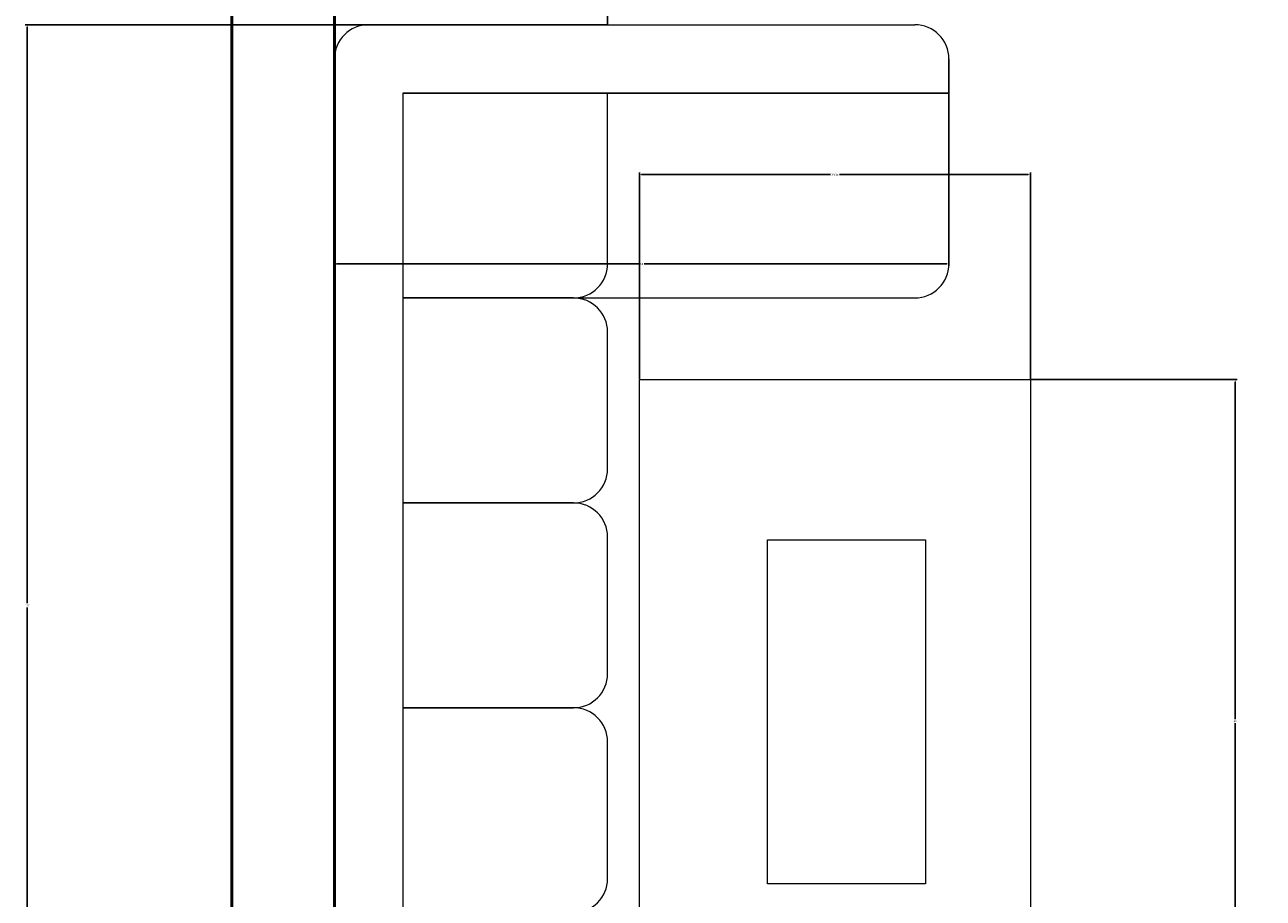
# Model space of a CAD drawing. Units: inches. Extents: x 2621 to 2849, y 2066 to 2463.
# Tile 2 of 28: x 2621 to 2729, y 2123 to 2199. Entities that reach past the tile are written whole.
import ezdxf

# ---------------------------------------------------------------- set-up
doc = ezdxf.new("R2010")
doc.units = ezdxf.units.IN
for name, color, linetype, lineweight in [('A-ANNO-DIMS', 2, 'Continuous', 18), ('A-FLOR-CASE', 9, 'Continuous', 25), ('A-FURN', 8, 'Continuous', 18), ('A-WALL', 7, 'Continuous', 50)]:
    doc.layers.add(name, color=color, linetype=linetype, lineweight=lineweight)
doc.styles.get("Standard").update_dxf_attribs({"font": 'arial.ttf'})
doc.dimstyles.get("Standard").update_dxf_attribs({"dimtxt": 0.18, "dimasz": 0.18, "dimexe": 0.18, "dimexo": 0.0625, "dimgap": 0.09, "dimtad": 0, "dimtih": 1, "dimtoh": 1, "dimdec": 4, "dimzin": 0, "dimdsep": 46, "dimtxsty": 'Standard', "dimcen": 0.09, "dimadec": 0, "dimazin": 0, "dimtfac": 1, "dimtdec": 4, "dimtofl": 0, "dimtmove": 0, "dimatfit": 3, "dimfxl": 1, "dimtolj": 1, "dimtzin": 0, "dimarcsym": 0})

# ---------------------------------------------------------------- blocks, each defined once
blk = doc.blocks.new('*D62')
at = {"layer": 'A-ANNO-DIMS', "color": 0, "lineweight": -2, "transparency": 16777216}
for p, q in [((2647.81, 2199.37), (2620.69, 2199.37)), ((2620.87, 2199.19), (2620.87, 2148.56)), ((2620.87, 2097.55), (2620.87, 2148.19)), ((2647.81, 2097.37), (2620.69, 2097.37))]:
    blk.add_line(p, q, dxfattribs=at)
at = {"layer": 'A-ANNO-DIMS', "color": 0, "transparency": 16777216}
for points in [[(2620.84, 2199.19), (2620.9, 2199.19), (2620.87, 2199.37)], [(2620.84, 2097.55), (2620.9, 2097.55), (2620.87, 2097.37)]]:
    blk.add_solid(points, dxfattribs=at)
at = {"layer": 'Defpoints', "color": 0, "transparency": 16777216}
for p in [(2620.87, 2199.37), (2647.87, 2199.37), (2647.87, 2097.37)]:
    blk.add_point(p, dxfattribs=at)
at = {"layer": 'A-ANNO-DIMS', "color": 0, "transparency": 16777216, "insert": (2620.87, 2148.37), "char_height": 0.18, "attachment_point": 5}
blk.add_mtext('\\A1;102', dxfattribs=at)
blk = doc.blocks.new('*D63')
at = {"layer": 'A-ANNO-DIMS', "color": 0, "lineweight": -2, "transparency": 16777216}
for p, q in [((2647.87, 2196.31), (2647.87, 2178.19)), ((2701.87, 2196.31), (2701.87, 2178.19)), ((2648.05, 2178.37), (2674.65, 2178.37)), ((2701.69, 2178.37), (2675.09, 2178.37))]:
    blk.add_line(p, q, dxfattribs=at)
at = {"layer": 'A-ANNO-DIMS', "color": 0, "transparency": 16777216}
for points in [[(2648.05, 2178.4), (2648.05, 2178.34), (2647.87, 2178.37)], [(2701.69, 2178.4), (2701.69, 2178.34), (2701.87, 2178.37)]]:
    blk.add_solid(points, dxfattribs=at)
at = {"layer": 'Defpoints', "color": 0, "transparency": 16777216}
for p in [(2647.87, 2196.37), (2701.87, 2196.37), (2647.87, 2178.37)]:
    blk.add_point(p, dxfattribs=at)
at = {"layer": 'A-ANNO-DIMS', "color": 0, "transparency": 16777216, "insert": (2674.87, 2178.37), "char_height": 0.18, "attachment_point": 5}
blk.add_mtext('\\A1;54', dxfattribs=at)
blk = doc.blocks.new('*D64')
at = {"layer": 'A-ANNO-DIMS', "color": 0, "lineweight": -2, "transparency": 16777216}
for p, q in [((2709.08, 2168.2), (2727.2, 2168.2)), ((2727.02, 2168.02), (2727.02, 2138.39)), ((2727.02, 2108.38), (2727.02, 2138.02)), ((2709.08, 2108.2), (2727.2, 2108.2))]:
    blk.add_line(p, q, dxfattribs=at)
at = {"layer": 'A-ANNO-DIMS', "color": 0, "transparency": 16777216}
for points in [[(2726.99, 2168.02), (2727.05, 2168.02), (2727.02, 2168.2)], [(2726.99, 2108.38), (2727.05, 2108.38), (2727.02, 2108.2)]]:
    blk.add_solid(points, dxfattribs=at)
at = {"layer": 'Defpoints', "color": 0, "transparency": 16777216}
for p in [(2709.02, 2168.2), (2709.02, 2108.2), (2727.02, 2108.2)]:
    blk.add_point(p, dxfattribs=at)
at = {"layer": 'A-ANNO-DIMS', "color": 0, "transparency": 16777216, "insert": (2727.02, 2138.2), "char_height": 0.18, "attachment_point": 5}
blk.add_mtext('\\A1;60', dxfattribs=at)
blk = doc.blocks.new('*D65')
at = {"layer": 'A-ANNO-DIMS', "color": 0, "lineweight": -2, "transparency": 16777216}
for p, q in [((2674.67, 2168.27), (2674.67, 2186.39)), ((2709.02, 2168.27), (2709.02, 2186.39)), ((2674.85, 2186.21), (2691.45, 2186.21)), ((2708.84, 2186.21), (2692.24, 2186.21))]:
    blk.add_line(p, q, dxfattribs=at)
at = {"layer": 'A-ANNO-DIMS', "color": 0, "transparency": 16777216}
for points in [[(2674.85, 2186.24), (2674.85, 2186.18), (2674.67, 2186.21)], [(2708.84, 2186.24), (2708.84, 2186.18), (2709.02, 2186.21)]]:
    blk.add_solid(points, dxfattribs=at)
at = {"layer": 'Defpoints', "color": 0, "transparency": 16777216}
for p in [(2709.02, 2186.21), (2674.67, 2168.2), (2709.02, 2168.2)]:
    blk.add_point(p, dxfattribs=at)
at = {"layer": 'A-ANNO-DIMS', "color": 0, "transparency": 16777216, "insert": (2691.85, 2186.21), "char_height": 0.18, "attachment_point": 5}
blk.add_mtext('\\A1;34.35', dxfattribs=at)

msp = doc.modelspace()

# ---------------------------------------------------------------- linework, layer by layer
at = {"layer": 'A-FLOR-CASE'}
for p, q in [((2671.8701, 2199.3746), (2671.8701, 2291.3746)), ((2647.8701, 2199.3746), (2671.8701, 2199.3746))]:
    msp.add_line(p, q, dxfattribs=at)
at = {"layer": 'A-FURN'}
for p, q in [((2650.8701, 2199.3746), (2698.8701, 2199.3746)), ((2647.8701, 2196.3746), (2647.8701, 2097.3746)), ((2701.8701, 2196.3746), (2701.8701, 2193.3746)), ((2653.8701, 2193.3746), (2701.8701, 2193.3746)), ((2653.8701, 2193.3746), (2653.8701, 2103.3746))]:
    msp.add_line(p, q, dxfattribs=at)
for points in [[(2653.8701, 2175.3746), (2668.8701, 2175.3746, 0.41421356), (2671.8701, 2178.3746), (2671.8701, 2193.3746), (2653.8701, 2193.3746)], [(2653.8701, 2157.3746), (2668.8701, 2157.3746, 0.41421356), (2671.8701, 2160.3746), (2671.8701, 2172.3746, 0.41421356), (2668.8701, 2175.3746), (2653.8701, 2175.3746)], [(2653.8701, 2139.3746), (2668.8701, 2139.3746, 0.41421356), (2671.8701, 2142.3746), (2671.8701, 2154.3746, 0.41421356), (2668.8701, 2157.3746), (2653.8701, 2157.3746)], [(2653.8701, 2121.3746), (2668.8701, 2121.3746, 0.41421356), (2671.8701, 2124.3746), (2671.8701, 2136.3746, 0.41421356), (2668.8701, 2139.3746), (2653.8701, 2139.3746)]]:
    msp.add_lwpolyline(points, format="xyb", close=True, dxfattribs=at)
for points in [[(2683.8701, 2193.3746), (2665.8701, 2193.3746)], [(2665.8701, 2175.3746), (2683.8701, 2175.3746)]]:
    msp.add_lwpolyline(points, dxfattribs=at)
msp.add_lwpolyline([(2683.8701, 2175.3746), (2698.8701, 2175.3746, 0.41421356), (2701.8701, 2178.3746), (2701.8701, 2193.3746), (2683.8701, 2193.3746)], format="xyb", dxfattribs=at)
for points in [[(2674.6703, 2168.2041), (2709.0205, 2168.2041), (2709.0205, 2108.2041), (2674.6703, 2108.2041)], [(2685.9183, 2154.1413), (2699.8172, 2154.1413), (2699.8172, 2123.9176), (2685.9183, 2123.9176)]]:
    msp.add_lwpolyline(points, close=True, dxfattribs=at)
for centre, start, end in [((2650.8701, 2196.3746), 90, 180), ((2698.8701, 2196.3746), 0, 90)]:
    msp.add_arc(centre, 3, start, end, dxfattribs=at)
at = {"layer": 'A-WALL'}
for p, q in [((2647.8701, 2199.3746), (2647.8701, 2315.3746)), ((2647.8701, 2093.3746), (2647.8701, 2199.3746))]:
    msp.add_line(p, q, dxfattribs=at)
msp.add_lwpolyline([(2761.8701, 2084.3746), (2638.8701, 2084.3746), (2638.8701, 2444.3746), (2830.8701, 2444.3746), (2830.8701, 2084.3746), (2797.8701, 2084.3746)], dxfattribs=at)

# ---------------------------------------------------------------- dimensions: what is measured, and where the dimension line sits
at = {"layer": 'A-ANNO-DIMS'}
for base, p1, p2, angle, picture, middle in [((2620.8666, 2199.3746), (2647.8701, 2097.3746), (2647.8701, 2199.3746), 90, '*D62', (2620.8666, 2148.3746)), ((2647.8701, 2178.3711), (2701.8701, 2196.3746), (2647.8701, 2196.3746), 180, '*D63', (2674.8701, 2178.3711)), ((2727.024, 2108.2041), (2709.0205, 2168.2041), (2709.0205, 2108.2041), 270, '*D64', (2727.024, 2138.2041))]:
    dim = msp.add_linear_dim(base=base, p1=p1, p2=p2, angle=angle, dimstyle='Standard', override={"dimdec": 0, "dimlfac": 1, "dimrnd": 0, "dimzin": 0, "dimdsep": 46, "dimlunit": 2}, dxfattribs=at)
    dim.commit()
    dim.dimension.update_dxf_attribs({"geometry": picture, "text_midpoint": middle})
dim = msp.add_linear_dim(base=(2709.0205, 2186.2076), p1=(2674.6703, 2168.2041), p2=(2709.0205, 2168.2041), dimstyle='Standard', override={"dimdec": 2, "dimlfac": 1, "dimrnd": 0, "dimzin": 0, "dimdsep": 46, "dimlunit": 2}, dxfattribs=at)
dim.commit()
dim.dimension.update_dxf_attribs({"geometry": '*D65', "text_midpoint": (2691.8454, 2186.2076)})

doc.saveas('drawing.dxf')
